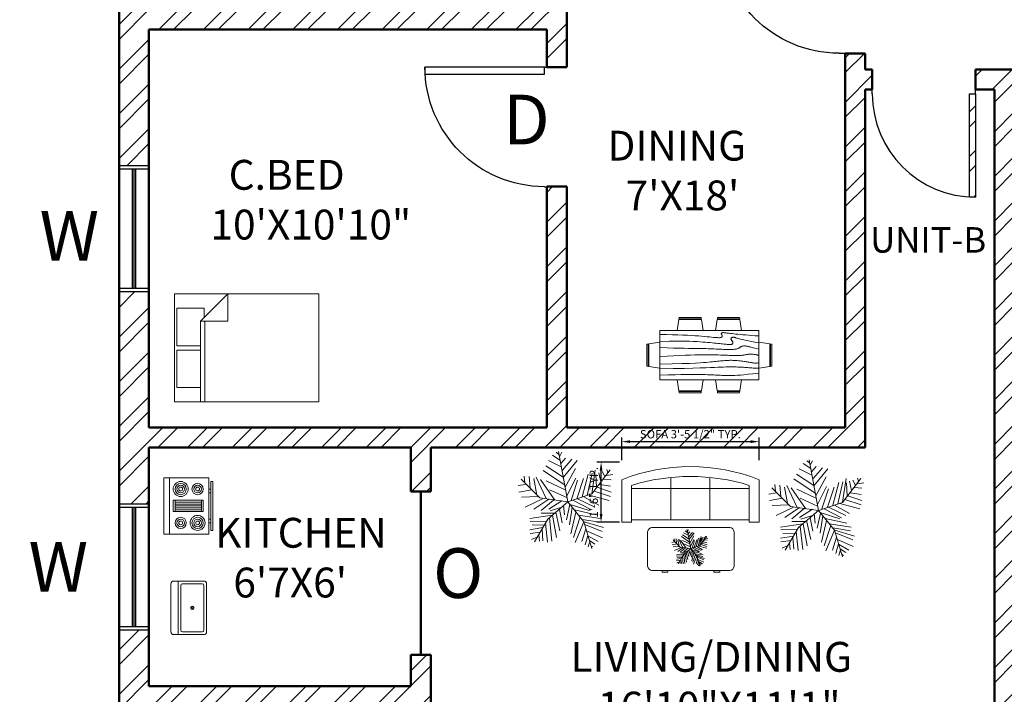
# Model space of a CAD drawing. Units: inches. Extents: x -31842 to -29388, y 18869 to 19743.
# Tile 6 of 12: x -30914 to -30617, y 19226 to 19429. Entities that reach past the tile are written whole.
import ezdxf

# ---------------------------------------------------------------- set-up
doc = ezdxf.new("R2010")
doc.units = ezdxf.units.IN
for name, color, linetype, lineweight in [('A-ANNO-DIMS', 2, 'Continuous', 18), ('A-ANNO-SYMB', 2, 'Continuous', 18), ('A-AREA-IDEN', 3, 'Continuous', 18), ('A-DOOR', 3, 'Continuous', 25), ('A-FLOR-FIXT', 8, 'Continuous', 18), ('A-FURN', 8, 'Continuous', 18), ('A-GLAZ', 4, 'Continuous', 25), ('A-WALL', 7, 'Continuous', 50), ('A-WALL-PATT', 8, 'Continuous', 13), ('L-PLNT', 3, 'Continuous', 13)]:
    doc.layers.add(name, color=color, linetype=linetype, lineweight=lineweight)
doc.styles.get("Standard").update_dxf_attribs({"font": 'arial.ttf'})
doc.dimstyles.new('ISO-25', dxfattribs={"dimtxt": 2.5, "dimasz": 2.5, "dimexe": 1.25, "dimexo": 0.625, "dimtad": 1, "dimdec": 0, "dimlunit": 3, "dimtxsty": 'Standard', "dimcen": 2.5, "dimadec": 0, "dimazin": 0, "dimtfac": 1, "dimtdec": 0, "dimtmove": 0, "dimatfit": 3, "dimfxl": 1, "dimarcsym": 0})

# ---------------------------------------------------------------- blocks, each defined once
blk = doc.blocks.new('*U8')
for p, q in [((0, 0), (0, -100)), ((750, 0), (750, -100))]:
    blk.add_line(p, q)
blk.add_lwpolyline([(0, 0), (0, 750), (43.75, 750), (43.75, 0)], close=True)
blk.add_arc((0, 0), 750, 0, 90)
blk = doc.blocks.new('Bed - Queen')
for p, q in [((0, -80.00003), (0, 0)), ((0, 0), (59.99999, 0)), ((59.99999, 0), (59.99999, -80.00003)), ((7.99999, -1.2), (28.79998, -1.2)), ((7.99999, -14.4), (7.99999, -1.2)), ((28.79998, -1.2), (28.79998, -14.4)), ((31.19999, -1.2), (51.99999, -1.2)), ((31.19999, -14.4), (31.19999, -1.2)), ((51.99999, -1.2), (51.99999, -16.4)), ((0, -14.4), (44.8, -14.4)), ((59.99999, -29.6), (44.8, -14.4)), ((44.8, -14.4), (44.8, -29.6)), ((44.8, -16.8), (0, -16.8)), ((51.99999, -16.4), (46.79936, -16.4)), ((44.8, -29.6), (59.99999, -29.6)), ((59.99999, -80.00003), (0, -80.00003))]:
    blk.add_line(p, q)
blk = doc.blocks.new('Range-Oven - 30 in top')
for p, q in [((0, -3), (30, -3)), ((12, -6), (18, -6)), ((13, -20), (13, -6)), ((14, -6), (14, -20)), ((15, -20), (15, -6)), ((16, -6), (16, -20)), ((17, -20), (17, -6)), ((18, -20), (12, -20)), ((6, -24), (6, -25)), ((8, -25), (8, -24)), ((22, -25), (22, -24)), ((24, -24), (24, -25))]:
    blk.add_line(p, q)
for points in [[(0, -24), (0, 0), (30, 0), (30, -24)], [(12, -21), (12, -5), (18, -5), (18, -21)], [(2, -26), (2, -25), (28, -25), (28, -26)]]:
    blk.add_lwpolyline(points, close=True)
for centre, radius in [((6, -9), 4), ((6, -9), 3), ((6, -9), 2), ((6, -9), 1), ((24, -9), 3), ((24, -9), 2), ((24, -9), 1), ((6, -18), 3), ((24, -18), 4), ((24, -18), 3), ((6, -18), 2), ((6, -18), 1), ((24, -18), 2), ((24, -18), 1)]:
    blk.add_circle(centre, radius)
blk = doc.blocks.new('Sink-single - 30 in top')
blk.add_line((-15, -3.999996), (15, -3.999996))
for points in [[(-13.5, 0), (13.5, 0)], [(-15, -18.499996), (-15, -1.5)], [(-12.5, -5.499996), (12.5, -5.499996)], [(15, -1.5), (15, -18.499996)], [(-13.5, -17.499996), (-13.5, -6.499996)], [(13.5, -6.499996), (13.5, -17.499996)], [(13.5, -19.999996), (-13.5, -19.999996)], [(12.5, -18.499996), (-12.5, -18.499996)]]:
    blk.add_lwpolyline(points)
for radius in [1, 0.5]:
    blk.add_circle((0, -11.999996), radius)
for centre, radius, start, end in [((-13.5, -1.5), 1.5, 90, 180), ((-12.5, -6.499996), 1, 90, 180), ((12.5, -6.499996), 1, 0, 90), ((13.5, -1.5), 1.5, 0, 90), ((-13.5, -18.499996), 1.5, 180, 270), ((-12.5, -17.499996), 1, 180, 270), ((12.5, -17.499996), 1, 270, 0), ((13.5, -18.499996), 1.5, 270, 0)]:
    blk.add_arc(centre, radius, start, end)
blk = doc.blocks.new('Desk - 30 x 60 in.')
for p, q in [((-26.999995, 0), (26.999995, 0)), ((-29.999995, -27), (-29.999995, -3)), ((29.999995, -3), (29.999995, -27)), ((26.999995, -30), (-26.999995, -30)), ((-20.000005, -30), (-20.000005, -31)), ((-20.000005, -31), (-16.000005, -31)), ((-16.000005, -31), (-16.000005, -30)), ((15.999995, -31), (15.999995, -30)), ((19.999995, -31), (15.999995, -31)), ((19.999995, -30), (19.999995, -31))]:
    blk.add_line(p, q)
for centre, start, end in [((-26.499995, -3.5), 98.1301, 171.8699), ((26.499995, -3.5), 8.130102, 81.8699), ((-26.499995, -26.5), 188.1301, 261.8699), ((26.499995, -26.5), 278.1301, 351.8699)]:
    blk.add_arc(centre, 3.535534, start, end)
blk = doc.blocks.new('Sofa - Roundback 7 ft.')
for p, q in [((-36.000027, -34), (-36.000027, -11.4696)), ((-12.00002, -32.4421), (-12.00003, -6.5971)), ((11.99997, -32.4421), (11.99998, -6.5971)), ((35.99998, -34), (35.99998, -11.4696)), ((-35.999844, -13.3819), (35.9998, -13.3819)), ((-36.000027, -32.4421), (35.99998, -32.4421))]:
    blk.add_line(p, q)
for points in [[(-36.000027, -34), (-42.000027, -34), (-42.000027, -8)], [(41.99998, -8), (41.99998, -34), (35.99998, -34)]]:
    blk.add_lwpolyline(points)
for centre, radius, start, end in [((0, -114.25), 114.25, 68.43141, 111.5686), ((-0.00001, -127.1968), 121.1968, 72.72033, 107.2797)]:
    blk.add_arc(centre, radius, start, end)
blk = doc.blocks.new('Dining Set - 36 x 72 in.')
for p, q in [((-22.2343, 26.00059), (-23.4847, 17.99762)), ((-22.2304, 26), (-5.7608, 26)), ((-22, 27.5), (-22.1562, 26.50042)), ((-5.8416, 26.5), (-22.1534, 26.5)), ((-22, 27.5), (-6, 27.5)), ((-5.8437, 26.49966), (-6, 27.5)), ((-4.5152, 17.99762), (-5.7655, 25.99926)), ((5.7657, 26.00059), (4.5153, 17.99762)), ((5.7696, 26), (22.2392, 26)), ((6, 27.5), (5.8438, 26.50042)), ((22.1584, 26.5), (5.8466, 26.5)), ((6, 27.5), (22, 27.5)), ((22.1563, 26.49966), (22, 27.5)), ((23.4848, 17.99762), (22.2345, 25.99926)), ((36, 18), (-36, 18)), ((-36, 18), (-36, -18)), ((36, -18), (36, 18)), ((-45.5, 8), (-44.5004, 8.15617)), ((-45.5, 8), (-45.5, -8)), ((-44.5, -8.15843), (-44.5, 8.15338)), ((-44.0006, 8.23428), (-35.9976, 9.48474)), ((-44, 8.23041), (-44, -8.23915)), ((44.0006, 8.23428), (35.9976, 9.48474)), ((44, 8.23041), (44, -8.23915)), ((44.5, -8.15843), (44.5, 8.15338)), ((45.5, 8), (44.5005, 8.15617)), ((45.5, 8), (45.5, -8)), ((-44.4997, -8.15631), (-45.5, -8)), ((-35.9976, -9.48476), (-43.9993, -8.2345)), ((35.9976, -9.48476), (43.9993, -8.2345)), ((44.4997, -8.15631), (45.5, -8)), ((-36, -18), (36, -18)), ((-22.2343, -26.0006), (-23.4847, -17.99762)), ((-4.5152, -17.99762), (-5.7655, -25.99928)), ((5.7657, -26.0006), (4.5153, -17.99762)), ((23.4848, -17.99762), (22.2345, -25.99928)), ((-22.2304, -26), (-5.7608, -26)), ((-22, -27.5), (-22.1562, -26.50044)), ((-5.8416, -26.5), (-22.1534, -26.5)), ((-22, -27.5), (-6, -27.5)), ((-5.8437, -26.49967), (-6, -27.5)), ((5.7696, -26), (22.2392, -26)), ((6, -27.5), (5.8438, -26.50044)), ((22.1584, -26.5), (5.8466, -26.5)), ((6, -27.5), (22, -27.5)), ((22.1563, -26.49967), (22, -27.5))]:
    blk.add_line(p, q)
for points in [[(-36, 15), (-31.1772, 14.97754), (-26.8079, 14.91406), (-22.8538, 14.81543), (-19.276, 14.6875), (-16.0362, 14.53613), (-13.0957, 14.36718), (-10.4159, 14.18652), (-7.9583, 14), (-5.6904, 13.81315), (-3.6035, 13.63021), (-1.6954, 13.45508), (0.0365, 13.29166), (1.5945, 13.14388), (2.9811, 13.01562), (4.1988, 12.9108), (5.25, 12.83333), (6.1393, 12.78613), (6.8802, 12.76823), (7.4883, 12.77767), (7.9792, 12.8125), (8.3685, 12.87077), (8.6719, 12.95052), (8.9049, 13.0498), (9.0833, 13.16666), (9.2205, 13.29899), (9.3216, 13.44401), (9.3895, 13.59879), (9.4271, 13.76041), (9.4373, 13.92594), (9.4232, 14.09245), (9.3875, 14.257), (9.3333, 14.41666), (9.2638, 14.56917), (9.1836, 14.71484), (9.0975, 14.85465), (9.0104, 14.98958), (8.9272, 15.1206), (8.8529, 15.2487), (8.7922, 15.37483), (8.75, 15.5), (8.7305, 15.62467), (8.7344, 15.74739), (8.7617, 15.86621), (8.8125, 15.97916), (8.8867, 16.08431), (8.9844, 16.17968), (9.1055, 16.26334), (9.25, 16.33333), (9.4189, 16.38802), (9.6172, 16.42708), (9.8506, 16.45052), (10.125, 16.45833), (10.4463, 16.45052), (10.8203, 16.42708), (11.2529, 16.38802), (11.75, 16.33333), (12.3184, 16.26318), (12.9694, 16.17838), (13.7151, 16.07991), (14.5677, 15.96875), (15.5395, 15.84586), (16.6426, 15.71224), (17.8893, 15.56884), (19.2917, 15.41666), (20.859, 15.25667), (22.5879, 15.08984), (24.4721, 14.91715), (26.5052, 14.73958), (28.6809, 14.5581), (30.9929, 14.3737), (33.4347, 14.18733), (36, 14)], [(-36, 10), (-28.9766, 10.14274), (-23.1725, 10.20442), (-18.4241, 10.19775), (-14.5677, 10.13541), (-11.4399, 10.03011), (-8.877, 9.89453), (-6.7154, 9.74137), (-4.7917, 9.58333), (-2.9698, 9.43082), (-1.2246, 9.28515), (0.4415, 9.14534), (2.026, 9.01041), (3.5266, 8.87939), (4.9408, 8.7513), (6.266, 8.62516), (7.5, 8.5), (8.6411, 8.37549), (9.6914, 8.2539), (10.6538, 8.13818), (11.5312, 8.03125), (12.3267, 7.93603), (13.043, 7.85547), (13.6831, 7.79248), (14.25, 7.75), (14.7471, 7.7303), (15.1797, 7.73307), (15.5537, 7.75732), (15.875, 7.80208), (16.1494, 7.86637), (16.3828, 7.94922), (16.5811, 8.04964), (16.75, 8.16666), (16.8944, 8.29915), (17.0143, 8.44531), (17.1089, 8.60319), (17.1771, 8.77083), (17.218, 8.94629), (17.2305, 9.1276), (17.2137, 9.31282), (17.1667, 9.5), (17.0895, 9.6875), (16.987, 9.875), (16.8649, 10.0625), (16.7292, 10.25), (16.5856, 10.4375), (16.4401, 10.625), (16.2985, 10.8125), (16.1667, 11), (16.05, 11.18733), (15.9518, 11.3737), (15.8752, 11.5581), (15.8229, 11.73958), (15.798, 11.91715), (15.8034, 12.08984), (15.842, 12.25667), (15.9167, 12.41666), (16.0295, 12.56836), (16.1784, 12.70833), (16.3605, 12.83268), (16.5729, 12.9375), (16.8127, 13.01888), (17.0768, 13.07291), (17.3625, 13.0957), (17.6667, 13.08333), (17.9894, 13.03312), (18.3418, 12.94726), (18.7382, 12.82918), (19.1927, 12.68229), (19.7195, 12.51001), (20.3327, 12.31575), (21.0465, 12.10294), (21.875, 11.875), (22.8357, 11.63354), (23.959, 11.37304), (25.2786, 11.08618), (26.8282, 10.76562), (28.6414, 10.40405), (30.752, 9.99414), (33.1936, 9.52856), (36, 9)], [(-36, 5.5), (-30.7157, 5.3348), (-26.069, 5.20963), (-21.9946, 5.11767), (-18.4271, 5.05208), (-15.3009, 5.00602), (-12.5508, 4.97265), (-10.1112, 4.94515), (-7.9167, 4.91666), (-5.909, 4.88167), (-4.0586, 4.83984), (-2.3429, 4.79215), (-0.7396, 4.73958), (0.7739, 4.6831), (2.22, 4.6237), (3.6213, 4.56233), (5, 4.5), (6.373, 4.43782), (7.7344, 4.3776), (9.0723, 4.32129), (10.375, 4.27083), (11.6309, 4.22819), (12.8281, 4.19531), (13.9551, 4.17415), (15, 4.16666), (15.954, 4.17448), (16.819, 4.19791), (17.6001, 4.23698), (18.3021, 4.29166), (18.9299, 4.36198), (19.4883, 4.44791), (19.9823, 4.54948), (20.4167, 4.66666), (20.7969, 4.79899), (21.1302, 4.94401), (21.4245, 5.09879), (21.6875, 5.26041), (21.9271, 5.42594), (22.1511, 5.59245), (22.3672, 5.757), (22.5834, 5.91666), (22.8065, 6.06868), (23.0404, 6.21093), (23.2879, 6.34147), (23.5521, 6.45833), (23.8358, 6.55957), (24.142, 6.64323), (24.4735, 6.70735), (24.8334, 6.75), (25.2235, 6.76969), (25.642, 6.76692), (26.0858, 6.74267), (26.5521, 6.69791), (27.0379, 6.63362), (27.5404, 6.55078), (28.0565, 6.45036), (28.5834, 6.33333), (29.1242, 6.19987), (29.7071, 6.04687), (30.3661, 5.87044), (31.1354, 5.66666), (32.0493, 5.43164), (33.142, 5.16146), (34.4475, 4.85221), (36, 4.5)], [(-36, -1), (-30.7915, -0.6591), (-26.0195, -0.38216), (-21.6519, -0.16284), (-17.6563, 0.00521), (-14.0005, 0.12833), (-10.6523, 0.21289), (-7.5796, 0.26522), (-4.75, 0.29166), (-2.134, 0.29793), (0.2878, 0.28711), (2.5317, 0.26163), (4.6146, 0.22396), (6.5529, 0.17651), (8.3633, 0.12174), (10.0623, 0.06209), (11.6667, 0), (13.1899, -0.06201), (14.6341, -0.1211), (15.9982, -0.17432), (17.2813, -0.21875), (18.4823, -0.25147), (19.6003, -0.26953), (20.6343, -0.27002), (21.5834, -0.25), (22.4481, -0.20768), (23.2357, -0.14584), (23.9549, -0.06836), (24.6146, 0.02083), (25.2235, 0.11784), (25.7904, 0.21875), (26.3241, 0.31966), (26.8334, 0.41666), (27.3265, 0.50618), (27.8099, 0.58593), (28.2894, 0.65397), (28.7709, 0.70833), (29.2601, 0.74707), (29.763, 0.76823), (30.2855, 0.76985), (30.8334, 0.75), (31.4088, 0.70784), (31.9994, 0.64713), (32.589, 0.57275), (33.1615, 0.48958), (33.7008, 0.4025), (34.1908, 0.3164), (34.6153, 0.23616), (34.9584, 0.16666), (35.2099, 0.11165), (35.3848, 0.07031), (35.504, 0.04069), (35.5886, 0.02083), (35.6594, 0.00879), (35.7377, 0.0026), (35.8442, 0.00032), (36, 0)], [(-36, -6.5), (-27.1843, -6.31267), (-20.084, -6.1263), (-14.469, -5.9419), (-10.1094, -5.76042), (-6.7752, -5.58285), (-4.2363, -5.41016), (-2.2629, -5.24333), (-0.625, -5.08334), (0.8708, -4.93099), (2.2715, -4.78646), (3.5872, -4.64974), (4.8281, -4.52084), (6.0046, -4.39974), (7.127, -4.28646), (8.2053, -4.18099), (9.25, -4.08334), (10.2705, -3.99382), (11.2734, -3.91407), (12.2647, -3.84603), (13.25, -3.79167), (14.2354, -3.75293), (15.2266, -3.73177), (16.2295, -3.73015), (17.25, -3.75), (18.2912, -3.79248), (19.3451, -3.85547), (20.4009, -3.93604), (21.4479, -4.03125), (22.4754, -4.13819), (23.4727, -4.25391), (24.4289, -4.37549), (25.3334, -4.5), (26.1785, -4.62492), (26.9694, -4.74935), (27.7145, -4.87281), (28.4219, -4.99479), (29.1, -5.11483), (29.7572, -5.23242), (30.4016, -5.34709), (31.0417, -5.45834), (31.6837, -5.56437), (32.3262, -5.65821), (32.9658, -5.73153), (33.599, -5.77604), (34.2224, -5.78345), (34.8327, -5.74545), (35.4264, -5.65373), (36, -5.5)], [(-36, -10), (-26.4022, -9.81299), (-18.4675, -9.62891), (-11.9839, -9.45069), (-6.7396, -9.28125), (-2.5226, -9.12354), (0.8789, -8.98047), (3.6769, -8.85498), (6.0833, -8.75), (8.2767, -8.66765), (10.3021, -8.60677), (12.1712, -8.56543), (13.8958, -8.54167), (15.4876, -8.53353), (16.9583, -8.53907), (18.3197, -8.55632), (19.5834, -8.58334), (20.7616, -8.61841), (21.8685, -8.66081), (22.9188, -8.71004), (23.9271, -8.76563), (24.9081, -8.82707), (25.8763, -8.89388), (26.8465, -8.96558), (27.8334, -9.04167), (28.8474, -9.12118), (29.8828, -9.20117), (30.93, -9.27824), (31.9792, -9.34896), (33.0205, -9.40991), (34.0443, -9.45768), (35.0407, -9.48885), (36, -9.5)], [(-36, -14.5), (-30.0881, -14.33513), (-25.0332, -14.21224), (-20.7312, -14.12647), (-17.0781, -14.07292), (-13.97, -14.04671), (-11.3027, -14.04297), (-8.9724, -14.05681), (-6.875, -14.08334), (-4.9224, -14.11833), (-3.0905, -14.16016), (-1.3709, -14.20785), (0.2448, -14.26042), (1.7647, -14.3169), (3.1973, -14.3763), (4.5507, -14.43767), (5.8333, -14.5), (7.0554, -14.5621), (8.235, -14.62175), (9.3922, -14.67652), (10.5469, -14.72396), (11.7192, -14.76164), (12.929, -14.78711), (14.1965, -14.79794), (15.5417, -14.79167), (16.9933, -14.76424), (18.6152, -14.70508), (20.4804, -14.60197), (22.6615, -14.44271), (25.2312, -14.21509), (28.2624, -13.9069), (31.8277, -13.50594), (36, -13)]]:
    blk.add_lwpolyline(points)
blk = doc.blocks.new('*U122')
for p, q in [((-258.7244, 1362.456), (-332.3336, 1421.4348)), ((0, 0), (-266.7, 1447.8)), ((-231.1146, 1315.2628), (-166.7002, 1421.4348)), ((-185.1152, 1008.5578), (-553.1612, 1185.4942)), ((-221.9198, 1197.3052), (-433.5526, 1338.8594)), ((-194.31, 1102.9442), (-65.4812, 1256.284)), ((-148.3106, 914.1968), (118.5418, 1220.9018)), ((-129.8956, 701.8528), (265.7602, 1185.4942)), ((-93.091, 489.5342), (-700.3796, 902.3858)), ((-129.8956, 713.6638), (-626.7704, 1032.1544)), ((-74.7014, 418.7444), (219.7608, 961.39)), ((685.8, 228.6), (1219.2, 914.4)), ((689.0258, 230.0224), (790.2448, 914.1968)), ((983.4626, 867.0036), (1066.2666, 725.4494)), ((1121.4862, 925.9824), (1149.0706, 831.6214)), ((-800.1, 114.3), (-1333.5, 647.7)), ((-1234.059, 536.7274), (-1252.4486, 737.2604)), ((-1105.2302, 725.4494), (-1077.6458, 395.1732)), ((-976.4268, 666.4706), (-884.4026, 194.6402)), ((-902.8176, 713.6638), (-617.5756, 100.2538)), ((-369.1382, 53.086), (-783.1836, 642.874)), ((-617.5756, 607.4918), (-74.7014, 347.98)), ((-28.6766, 171.0436), (228.9556, 678.2816)), ((100.1268, 41.275), (284.1498, 619.2774)), ((256.5654, 88.4682), (449.7832, 666.4706)), ((412.9786, 147.447), (587.8068, 796.2392)), ((560.197, 182.8292), (698.2206, 819.8358)), ((808.6344, 784.4282), (827.0494, 418.7444)), ((891.4384, 831.6214), (946.658, 572.1096)), ((1029.462, 654.685), (1241.0948, 631.0884)), ((1112.2914, 760.8316), (1296.3144, 784.4282)), ((-1206.4492, 501.3198), (-1418.082, 465.9376)), ((-1031.621, 347.98), (-1399.667, 277.1902)), ((-525.5514, 347.98), (-28.6766, 123.8504)), ((753.4148, 312.5978), (1222.6798, 159.2326)), ((845.439, 418.7444), (1241.0948, 277.1902)), ((919.0482, 501.3198), (1222.6798, 454.152)), ((-847.598, 159.2326), (-1326.0578, 135.636)), ((-718.7946, 88.4682), (-1215.644, -147.447)), ((-543.9664, 76.6572), (-967.2066, -206.4512)), ((0, 0), (-800.1, 114.3)), ((-405.9428, 53.086), (-764.794, -241.8334)), ((0, 0), (-571.5, -495.3)), ((-166.7002, 29.4894), (-543.9664, -206.4512)), ((0, 0), (685.8, 228.6)), ((0, 0), (457.2, -571.5)), ((164.5412, 41.275), (661.416, -218.2368)), ((284.1498, 88.4682), (781.0246, -147.447)), ((458.978, 147.447), (891.4384, -88.4682)), ((615.4166, 194.6402), (1185.8752, 41.275)), ((-166.7002, -147.447), (-507.1618, -253.619)), ((-240.3094, -218.2368), (-157.5054, -595.7062)), ((-120.7008, -88.4682), (-93.091, -371.5766)), ((63.3222, -76.6826), (-37.8714, -513.1308)), ((44.9326, -64.897), (615.4166, -241.8334)), ((127.7366, -159.258), (54.1274, -654.685)), ((192.151, -230.0224), (817.8292, -371.5766)), ((-442.7474, -383.3876), (-1086.8406, -477.7486)), ((-617.5756, -548.5384), (-1077.6458, -560.324)), ((-571.5, -495.3), (-952.5, -1143)), ((-387.5278, -324.4088), (-764.794, -324.4088)), ((-525.5514, -465.963), (-451.9422, -1126.5408)), ((-433.5526, -383.3876), (-323.1134, -1020.3688)), ((-341.5284, -289.0012), (-221.9198, -831.6214)), ((228.9556, -289.0012), (90.932, -914.1968)), ((357.759, -430.5554), (164.5412, -1020.3688)), ((311.7596, -383.3876), (937.4378, -477.7486)), ((412.9786, -501.3452), (919.0482, -583.9206)), ((-718.7946, -737.2604), (-1086.8406, -796.2392)), ((-681.9646, -666.496), (-1022.4262, -654.685)), ((-737.1842, -784.4536), (-709.5744, -1114.7298)), ((-635.9652, -607.5172), (-580.771, -1150.1374)), ((458.978, -572.1096), (210.5406, -1161.923)), ((514.1976, -772.6426), (403.7838, -1138.3264)), ((457.2, -571.5), (685.8, -1333.5)), ((468.1982, -572.1096), (1029.462, -737.2604)), ((486.5878, -642.8994), (983.4626, -843.4324)), ((541.8074, -831.6214), (992.6574, -1032.1544)), ((-783.1836, -867.029), (-1077.6458, -902.4112)), ((-875.2078, -1008.5832), (-1040.8412, -1079.3476)), ((-829.2084, -937.7934), (-810.7934, -1126.5408)), ((578.612, -961.39), (495.7826, -1232.7128)), ((578.612, -973.1756), (873.0488, -1138.3264)), ((624.6114, -1102.9442), (781.0246, -1209.1162)), ((624.6114, -1161.923), (587.8068, -1291.6916)), ((679.8056, -1268.095), (716.6102, -1291.6916))]:
    blk.add_line(p, q)
blk = doc.blocks.new('WIN-3FT')
for p, q in [((0, 36), (9, 36)), ((4, 0), (4, 36)), ((4.5, 0), (4.5, 36)), ((5, 0), (5, 36)), ((0, 0), (9, 0))]:
    blk.add_line(p, q)
blk = doc.blocks.new('*D255')
at = {"layer": 'A-ANNO-DIMS', "color": 0, "lineweight": -2, "transparency": 16777216}
for p, q in [((-30732.8, 19296.13), (-30732.8, 19302.97)), ((-30691.37, 19296.13), (-30691.37, 19302.97)), ((-30730.3, 19301.72), (-30693.87, 19301.72))]:
    blk.add_line(p, q, dxfattribs=at)
at = {"layer": 'A-ANNO-DIMS', "color": 0, "transparency": 16777216}
for points in [[(-30730.3, 19302.14), (-30730.3, 19301.31), (-30732.8, 19301.72)], [(-30693.87, 19302.14), (-30693.87, 19301.31), (-30691.37, 19301.72)]]:
    blk.add_solid(points, dxfattribs=at)
at = {"layer": 'Defpoints', "color": 0, "transparency": 16777216}
for p in [(-30691.37, 19301.72), (-30732.8, 19295.51), (-30691.37, 19295.51)]:
    blk.add_point(p, dxfattribs=at)
at = {"layer": 'A-ANNO-DIMS', "color": 0, "transparency": 16777216, "insert": (-30712.09, 19303.64), "char_height": 2.5, "attachment_point": 5}
blk.add_mtext('SOFA 3\'-5 1/2" TYP.', dxfattribs=at)
blk = doc.blocks.new('*D256')
at = {"layer": 'A-ANNO-DIMS', "color": 0, "lineweight": -2, "transparency": 16777216}
for p, q in [((-30733.43, 19295.51), (-30740.27, 19295.51)), ((-30739.02, 19279.92), (-30739.02, 19293.01)), ((-30733.43, 19277.42), (-30740.27, 19277.42))]:
    blk.add_line(p, q, dxfattribs=at)
at = {"layer": 'A-ANNO-DIMS', "color": 0, "transparency": 16777216}
for points in [[(-30739.44, 19293.01), (-30738.6, 19293.01), (-30739.02, 19295.51)], [(-30739.44, 19279.92), (-30738.6, 19279.92), (-30739.02, 19277.42)]]:
    blk.add_solid(points, dxfattribs=at)
at = {"layer": 'Defpoints', "color": 0, "transparency": 16777216}
for p in [(-30739.02, 19295.51), (-30732.8, 19295.51), (-30732.8, 19277.42)]:
    blk.add_point(p, dxfattribs=at)
at = {"layer": 'A-ANNO-DIMS', "color": 0, "transparency": 16777216, "insert": (-30740.92, 19286.47), "char_height": 2.5, "attachment_point": 5, "rotation": 90}
blk.add_mtext('1\'-6" TYP.', dxfattribs=at)

msp = doc.modelspace()

# ---------------------------------------------------------------- hatches: boundary and pattern name
at = {"layer": 'A-WALL-PATT'}
h = msp.add_hatch(dxfattribs=at)
h.set_pattern_fill('ANSI32', color=256)
h.paths.add_polyline_path([(-30352.39, 19656.96), (-30487.39, 19656.96), (-30487.39, 19614.96), (-30510.39, 19614.96), (-30510.39, 19605.96), (-30487.39, 19605.96), (-30487.39, 19558.38), (-30481.39, 19558.38), (-30481.39, 19605.96), (-30469.68, 19605.96), (-30469.68, 19614.96), (-30481.39, 19614.96), (-30481.39, 19650.96), (-30361.39, 19650.96), (-30361.39, 19614.96), (-30445.68, 19614.96), (-30445.68, 19605.96), (-30361.39, 19605.96), (-30361.39, 19564.96), (-30352.39, 19564.96)])
h.paths.add_polyline_path([(-30548.39, 19614.96), (-30599.39, 19614.96), (-30599.39, 19605.96), (-30577.39, 19605.96), (-30577.39, 19457.87), (-30571.39, 19457.87), (-30571.39, 19491.96), (-30560.76, 19491.96), (-30560.76, 19497.96), (-30571.39, 19497.96), (-30571.39, 19605.96), (-30548.39, 19605.96)])
h.paths.add_polyline_path([(-30637.39, 19614.96), (-30688.39, 19614.96), (-30688.39, 19605.96), (-30665.39, 19605.96), (-30665.39, 19497.96), (-30682.48, 19497.96), (-30682.48, 19491.96), (-30665.39, 19491.96), (-30665.39, 19454.79), (-30662.43, 19454.79), (-30659.39, 19454.79), (-30659.39, 19605.96), (-30637.39, 19605.96)])
h.paths.add_polyline_path([(-30789.63, 19614.96), (-30875.39, 19614.96), (-30875.39, 19650.96), (-30755.39, 19650.96), (-30755.39, 19614.96), (-30765.63, 19614.96), (-30765.63, 19605.96), (-30755.39, 19605.96), (-30755.39, 19550.68), (-30749.39, 19550.68), (-30749.39, 19605.96), (-30726.39, 19605.96), (-30726.39, 19614.96), (-30749.39, 19614.96), (-30749.39, 19656.96), (-30884.39, 19656.96), (-30884.39, 19564.96), (-30875.39, 19564.96), (-30875.39, 19605.96), (-30789.63, 19605.96)])
h.paths.add_polyline_path([(-30749.39, 19491.96), (-30736.92, 19491.96), (-30736.92, 19494.96), (-30682.48, 19494.96), (-30682.48, 19497.96), (-30665.39, 19497.96), (-30665.39, 19605.96), (-30688.39, 19605.96), (-30749.39, 19605.96), (-30749.39, 19550.68), (-30755.39, 19550.68), (-30757.34, 19550.71, 0.39722), (-30793.34, 19516.76), (-30757.34, 19516.76), (-30757.34, 19514.65), (-30793.4, 19514.65), (-30793.4, 19516.76), (-30793.34, 19516.76, -0.39722), (-30757.34, 19550.71), (-30755.39, 19550.71), (-30755.39, 19605.96), (-30765.63, 19605.96), (-30765.63, 19613.66), (-30767.03, 19613.66), (-30767.03, 19637.62, 0.397344), (-30789.63, 19613.65), (-30789.63, 19605.96), (-30875.39, 19605.96), (-30875.39, 19564.96), (-30875.39, 19485.96), (-30873.79, 19485.96), (-30873.79, 19479.96), (-30873.79, 19479.35, 0.39722), (-30851.19, 19455.39), (-30851.19, 19479.35), (-30849.79, 19479.35), (-30849.79, 19455.34), (-30851.19, 19455.34), (-30851.19, 19455.39, -0.39722), (-30873.79, 19479.35), (-30873.79, 19479.96), (-30875.39, 19479.96), (-30875.39, 19431.96), (-30848.39, 19431.96), (-30848.39, 19468.96), (-30842.39, 19468.96), (-30842.39, 19479.96), (-30755.39, 19479.96), (-30755.39, 19470.97), (-30749.39, 19470.97)])
h.paths.add_polyline_path([(-30738.39, 19585.51), (-30738.39, 19586.08), (-30736.12, 19586.08), (-30736.12, 19586.65), (-30739.53, 19586.65), (-30739.53, 19600.27), (-30722.5, 19600.27), (-30722.5, 19586.65), (-30725.91, 19586.65), (-30725.91, 19586.08), (-30723.64, 19586.08), (-30723.64, 19585.51)], flags=16)
h.paths.add_polyline_path([(-30737.83, 19590.05, -1), (-30734.42, 19590.05, -1)], flags=16)
h.paths.add_polyline_path([(-30737.26, 19590.05, -1), (-30734.99, 19590.05, -1)], flags=0)
h.paths.add_polyline_path([(-30732.72, 19588.35), (-30732.72, 19597.43), (-30729.31, 19597.43), (-30729.31, 19588.35)], flags=16)
h.paths.add_polyline_path([(-30736.69, 19590.05, -1), (-30735.56, 19590.05, -1)], flags=0)
h.paths.add_polyline_path([(-30732.15, 19588.92), (-30732.15, 19596.86), (-30729.88, 19596.86), (-30729.88, 19588.92)], flags=0)
h.paths.add_polyline_path([(-30728.18, 19590.05, -1), (-30723.64, 19590.05, -1)], flags=0)
h.paths.add_polyline_path([(-30727.61, 19590.05, -1), (-30724.2, 19590.05, -1)], flags=0)
h.paths.add_polyline_path([(-30727.04, 19590.05, -1), (-30724.77, 19590.05, -1)], flags=0)
h.paths.add_polyline_path([(-30726.47, 19590.05, -1), (-30725.34, 19590.05, -1)], flags=0)
h.paths.add_polyline_path([(-30738.39, 19595.16, -1), (-30733.85, 19595.16, -1)], flags=16)
h.paths.add_polyline_path([(-30737.83, 19595.16, -1), (-30734.42, 19595.16, -1)], flags=0)
h.paths.add_polyline_path([(-30737.26, 19595.16, -1), (-30734.99, 19595.16, -1)], flags=0)
h.paths.add_polyline_path([(-30736.69, 19595.16, -1), (-30735.56, 19595.16, -1)], flags=0)
h.paths.add_polyline_path([(-30727.61, 19595.16, -1), (-30724.2, 19595.16, -1)], flags=0)
h.paths.add_polyline_path([(-30727.04, 19595.16, -1), (-30724.77, 19595.16, -1)], flags=0)
h.paths.add_polyline_path([(-30707.55, 19587.34, -0.414214), (-30708.36, 19588.14), (-30708.36, 19597.29, -0.414214), (-30707.55, 19598.09), (-30693.03, 19598.09, -0.414214), (-30692.23, 19597.29), (-30692.23, 19588.14, -0.414214), (-30693.03, 19587.34)], flags=16)
h.paths.add_polyline_path([(-30726.47, 19595.16, -1), (-30725.34, 19595.16, -1)], flags=0)
h.paths.add_polyline_path([(-30827.74, 19570.11), (-30871.22, 19570.11), (-30871.22, 19602.72), (-30827.74, 19602.72)], flags=16)
h.paths.add_polyline_path([(-30707.01, 19588.14, -0.414214), (-30707.55, 19588.68), (-30707.55, 19594.6, -0.414214), (-30707.01, 19595.13), (-30693.57, 19595.13, -0.414214), (-30693.03, 19594.6), (-30693.03, 19588.68, -0.414214), (-30693.57, 19588.14)], flags=0)
h.paths.add_polyline_path([(-30700.02, 19591.64, -1), (-30700.56, 19591.64, -1)], flags=0)
h.paths.add_polyline_path([(-30863.39, 19594.46), (-30863.39, 19574.46), (-30870.57, 19574.46), (-30870.57, 19585.76), (-30863.39, 19585.76), (-30863.39, 19587.07), (-30870.57, 19587.07), (-30870.57, 19598.37), (-30862.31, 19598.37), (-30862.31, 19595.55), (-30855.13, 19602.72), (-30855.13, 19594.46)], flags=0)
h.paths.add_polyline_path([(-30755.39, 19514.65), (-30757.34, 19514.65), (-30793.4, 19514.65), (-30793.4, 19516.76), (-30793.34, 19516.76, -0.39722), (-30757.34, 19550.71), (-30755.39, 19550.71), (-30755.39, 19605.96), (-30765.63, 19605.96), (-30765.63, 19613.66), (-30767.03, 19613.66), (-30767.03, 19637.62, 0.397344), (-30789.63, 19613.65), (-30789.63, 19605.96), (-30875.39, 19605.96), (-30875.39, 19564.96), (-30875.39, 19485.96), (-30873.79, 19485.96), (-30873.79, 19479.96), (-30873.79, 19479.35, 0.39722), (-30851.19, 19455.39), (-30851.19, 19479.35), (-30849.79, 19479.35), (-30849.79, 19479.96), (-30849.79, 19479.96), (-30849.79, 19485.96), (-30755.39, 19485.96)], flags=16)
h.paths.add_polyline_path([(-30665.39, 19605.96), (-30688.39, 19605.96), (-30749.39, 19605.96), (-30749.39, 19550.68), (-30755.39, 19550.68), (-30757.34, 19550.71, 0.39722), (-30793.34, 19516.76), (-30757.34, 19516.76), (-30757.34, 19514.65), (-30755.39, 19514.65), (-30755.39, 19514.68), (-30749.39, 19514.68), (-30749.39, 19497.96), (-30736.92, 19497.96), (-30736.92, 19494.96), (-30682.48, 19494.96), (-30682.48, 19497.96), (-30665.39, 19497.96)], flags=17)
h.paths.add_polyline_path([(-30749.39, 19446.97), (-30755.39, 19446.97), (-30755.39, 19431.96), (-30842.39, 19431.96), (-30842.39, 19442.96), (-30848.39, 19442.96), (-30848.39, 19431.96), (-30875.39, 19431.96), (-30875.39, 19479.96), (-30873.79, 19479.96), (-30873.79, 19482.55), (-30873.79, 19485.96), (-30875.39, 19485.96), (-30875.39, 19526.96), (-30884.39, 19526.96), (-30884.39, 19384.96), (-30875.39, 19384.96), (-30875.39, 19425.96), (-30755.39, 19425.96), (-30755.39, 19414.67), (-30751.3, 19414.67), (-30749.39, 19414.62)])
h.paths.add_polyline_path([(-30848.39, 19468.96), (-30848.39, 19479.96), (-30849.79, 19479.96), (-30849.79, 19479.35), (-30849.79, 19455.34), (-30851.19, 19455.34), (-30851.19, 19455.39, -0.39722), (-30873.79, 19479.35), (-30873.79, 19479.96), (-30875.39, 19479.96), (-30875.39, 19431.96), (-30848.39, 19431.96), (-30848.39, 19442.96)], flags=17)
h.paths.add_polyline_path([(-30659.39, 19407.96), (-30657.22, 19407.96), (-30657.22, 19413.96), (-30659.39, 19413.96), (-30659.39, 19418.79), (-30665.39, 19418.79), (-30665.39, 19305.96), (-30749.39, 19305.96), (-30749.39, 19378.62), (-30755.39, 19378.62), (-30755.39, 19305.96), (-30875.39, 19305.96), (-30875.39, 19346.96), (-30884.39, 19346.96), (-30884.39, 19282.96), (-30875.39, 19282.96), (-30875.39, 19299.96), (-30796.39, 19299.96), (-30796.39, 19286.68), (-30790.39, 19286.68), (-30790.39, 19299.96), (-30659.39, 19299.96)])
h.paths.add_polyline_path([(-30352.39, 19346.96), (-30361.39, 19346.96), (-30361.39, 19305.96), (-30481.39, 19305.96), (-30481.39, 19380.1), (-30487.39, 19380.1), (-30487.39, 19305.96), (-30571.39, 19305.96), (-30571.39, 19421.87), (-30577.39, 19421.87), (-30577.39, 19413.96), (-30579.53, 19413.96), (-30579.53, 19407.96), (-30577.39, 19407.96), (-30577.39, 19299.96), (-30446.39, 19299.96), (-30446.39, 19291.76), (-30440.39, 19291.76), (-30440.39, 19299.96), (-30361.39, 19299.96), (-30361.39, 19282.96), (-30352.39, 19282.96)])
h.paths.add_polyline_path([(-30481.39, 19449.62), (-30484.39, 19449.62), (-30487.39, 19449.62), (-30487.39, 19416.1), (-30481.39, 19416.1), (-30481.39, 19425.96), (-30361.39, 19425.96), (-30361.39, 19384.96), (-30352.39, 19384.96), (-30352.39, 19526.96), (-30361.39, 19526.96), (-30361.39, 19485.96), (-30363.32, 19485.96), (-30363.32, 19479.96), (-30361.39, 19479.96), (-30361.39, 19431.96), (-30388.39, 19431.96), (-30388.39, 19442.96), (-30394.39, 19442.96), (-30394.39, 19431.96), (-30481.39, 19431.96)])
h.paths.add_polyline_path([(-30387.32, 19482.76), (-30387.32, 19485.96), (-30481.39, 19485.96), (-30481.39, 19522.38), (-30487.39, 19522.38), (-30487.39, 19497.96), (-30500.08, 19497.96), (-30500.08, 19491.96), (-30487.39, 19491.96), (-30487.39, 19473.62), (-30481.39, 19473.62), (-30481.39, 19479.96), (-30394.39, 19479.96), (-30394.39, 19468.96), (-30388.39, 19468.96), (-30388.39, 19479.96), (-30387.32, 19479.96)])
h.paths.add_polyline_path([(-30626.04, 19413.96), (-30610.58, 19413.96), (-30610.58, 19407.24), (-30608.81, 19407.24), (-30608.81, 19376.14), (-30610.63, 19376.14), (-30610.63, 19407.96), (-30614.39, 19407.96), (-30614.39, 19173.96), (-30532.79, 19173.96), (-30532.79, 19167.96), (-30532.79, 19166.59), (-30532.79, 19167.96), (-30614.39, 19167.96), (-30614.39, 19023.96), (-30568.89, 19023.96), (-30568.89, 19014.96), (-30666.89, 19014.96), (-30666.89, 19018.96), (-30702.89, 19018.96), (-30702.89, 19019.96), (-30666.89, 19019.96), (-30666.89, 19023.96), (-30620.39, 19023.96), (-30620.39, 19167.96), (-30707.45, 19167.96), (-30707.45, 19166.65, -0.39722), (-30741.49, 19130.57), (-30741.49, 19130.51), (-30743.6, 19130.51), (-30743.6, 19166.65), (-30741.49, 19166.65), (-30741.49, 19130.57, 0.407721), (-30707.48, 19167.96), (-30707.53, 19167.96), (-30707.53, 19173.96), (-30620.39, 19173.96), (-30620.39, 19407.96), (-30626.04, 19407.96), (-30626.04, 19406.62), (-30626.04, 19375.45), (-30627.86, 19375.45), (-30627.86, 19406.62), (-30626.04, 19406.62), (-30626.04, 19407.96), (-30626.04, 19407.96)])
h.paths.add_polyline_path([(-30481.39, 19167.96), (-30478.24, 19167.96), (-30478.24, 19173.96), (-30487.39, 19173.96), (-30496.79, 19173.96), (-30496.79, 19167.96), (-30487.39, 19167.96), (-30487.39, 19023.96), (-30531.89, 19023.96), (-30531.89, 19014.96), (-30449.39, 19014.96), (-30449.39, 19023.96), (-30481.39, 19023.96)])
h.paths.add_polyline_path([(-30322.39, 19173.96), (-30343.77, 19173.96), (-30343.77, 19167.96), (-30328.39, 19167.96), (-30328.39, 19023.96), (-30373.39, 19023.96), (-30373.39, 19076.96), (-30379.39, 19076.96), (-30379.39, 19023.96), (-30411.39, 19023.96), (-30411.39, 19014.96), (-30322.39, 19014.96)])
h.paths.add_polyline_path([(-30367.77, 19173.96), (-30440.39, 19173.96), (-30440.39, 19191.96), (-30446.39, 19191.96), (-30446.39, 19173.96), (-30449.24, 19173.96), (-30449.24, 19167.96), (-30379.39, 19167.96), (-30379.39, 19114.96), (-30373.39, 19114.96), (-30373.39, 19167.96), (-30367.77, 19167.96)])
h.paths.add_polyline_path([(-30857.39, 19167.96), (-30814.74, 19167.96), (-30787.91, 19167.96), (-30787.91, 19173.96), (-30790.39, 19173.96), (-30790.39, 19191.02), (-30796.39, 19191.02), (-30796.39, 19173.96), (-30814.74, 19173.96), (-30871.78, 19173.96), (-30871.78, 19167.96), (-30863.39, 19167.96), (-30863.39, 19114.96), (-30857.39, 19114.96)])
h.paths.add_polyline_path([(-30857.39, 19076.96), (-30863.39, 19076.96), (-30863.39, 19023.96), (-30908.39, 19023.96), (-30908.39, 19167.96), (-30895.78, 19167.96), (-30895.78, 19173.96), (-30914.39, 19173.96), (-30914.39, 19014.96), (-30825.39, 19014.96), (-30825.39, 19023.96), (-30857.39, 19023.96)])
h.paths.add_polyline_path([(-30758.91, 19173.96), (-30743.53, 19173.96), (-30743.53, 19167.96), (-30743.6, 19166.65), (-30741.49, 19166.65), (-30741.49, 19130.51), (-30743.6, 19130.51), (-30743.6, 19166.65), (-30743.6, 19167.96), (-30749.39, 19167.96), (-30749.39, 19023.96), (-30702.89, 19023.96), (-30702.89, 19019.46), (-30666.89, 19019.46), (-30666.89, 19018.96), (-30702.89, 19018.96), (-30702.89, 19014.96), (-30788.39, 19014.96), (-30788.39, 19018.96), (-30824.39, 19018.96), (-30824.39, 19019.96), (-30788.39, 19019.96), (-30788.39, 19023.96), (-30755.39, 19023.96), (-30755.39, 19167.96), (-30758.91, 19167.96), (-30758.91, 19166.97), (-30758.91, 19137.97), (-30760.6, 19137.97), (-30760.6, 19166.97), (-30758.91, 19166.97), (-30758.91, 19167.96), (-30758.91, 19167.96)])
h.paths.add_polyline_path([(-30790.39, 19237.4), (-30796.39, 19237.4), (-30796.39, 19227.96), (-30875.39, 19227.96), (-30875.39, 19244.96), (-30884.39, 19244.96), (-30884.39, 19210.96), (-30875.39, 19210.96), (-30875.39, 19221.96), (-30796.39, 19221.96), (-30796.39, 19215.02), (-30793.87, 19215.02), (-30790.39, 19215.02)])
h.paths.add_polyline_path([(-30352.39, 19244.96), (-30361.39, 19244.96), (-30361.39, 19227.96), (-30440.39, 19227.96), (-30440.39, 19236.96), (-30446.39, 19236.96), (-30446.39, 19215.96), (-30440.39, 19215.96), (-30440.39, 19221.96), (-30361.39, 19221.96), (-30361.39, 19210.96), (-30352.39, 19210.96)])
h.paths.add_polyline_path([(-30788.99, 19602.36), (-30766.36, 19602.36), (-30766.36, 19633.27), (-30788.99, 19633.27)], flags=24)
h.paths.add_polyline_path([(-30871.43, 19460.05), (-30848.8, 19460.05), (-30848.8, 19490.96), (-30871.43, 19490.96)], flags=24)
h.paths.add_polyline_path([(-30778.82, 19519.23), (-30756.18, 19519.23), (-30756.18, 19550.14), (-30778.82, 19550.14)], flags=24)
h.paths.add_polyline_path([(-30741.54, 19533.68), (-30681.86, 19533.68), (-30681.86, 19567.23), (-30741.54, 19567.23)], flags=24)
h.paths.add_polyline_path([(-30866.65, 19526.15), (-30802.54, 19526.15), (-30802.54, 19559.73), (-30866.65, 19559.73)], flags=8)

# ---------------------------------------------------------------- linework, layer by layer
at = {"layer": 'A-GLAZ'}
for p, q in [((-30884.39, 19384.96), (-30875.39, 19384.96)), ((-30884.39, 19346.96), (-30875.39, 19346.96)), ((-30884.39, 19282.96), (-30875.39, 19282.96)), ((-30884.39, 19244.96), (-30875.39, 19244.96))]:
    msp.add_line(p, q, dxfattribs=at)
at = {"layer": 'A-WALL'}
for p, q in [((-30884.39, 19173.96), (-30884.39, 19656.96)), ((-30749.39, 19414.62), (-30749.39, 19446.97)), ((-30875.39, 19425.96), (-30755.39, 19425.96)), ((-30875.39, 19305.96), (-30875.39, 19425.96)), ((-30755.39, 19414.62), (-30755.39, 19425.96)), ((-30665.39, 19305.96), (-30665.39, 19418.79)), ((-30665.39, 19418.79), (-30659.39, 19418.79)), ((-30659.39, 19413.96), (-30659.39, 19418.79)), ((-30755.39, 19414.62), (-30749.39, 19414.62)), ((-30659.39, 19413.96), (-30657.22, 19413.96)), ((-30657.22, 19407.96), (-30657.22, 19413.96)), ((-30626.04, 19407.96), (-30626.04, 19413.96)), ((-30626.04, 19413.96), (-30610.58, 19413.96)), ((-30659.39, 19299.96), (-30659.39, 19407.96)), ((-30659.39, 19407.96), (-30657.22, 19407.96)), ((-30626.04, 19407.96), (-30620.39, 19407.96)), ((-30620.39, 19173.96), (-30620.39, 19407.96)), ((-30755.39, 19305.96), (-30755.39, 19378.62)), ((-30755.39, 19378.62), (-30749.39, 19378.62)), ((-30749.39, 19305.96), (-30749.39, 19378.62)), ((-30875.39, 19305.96), (-30755.39, 19305.96)), ((-30749.39, 19305.96), (-30665.39, 19305.96)), ((-30875.39, 19299.96), (-30796.39, 19299.96)), ((-30875.39, 19227.96), (-30875.39, 19299.96)), ((-30796.39, 19286.68), (-30796.39, 19299.96)), ((-30790.39, 19299.96), (-30659.39, 19299.96)), ((-30790.39, 19286.68), (-30790.39, 19299.96)), ((-30796.39, 19286.68), (-30790.39, 19286.68)), ((-30793.39, 19286.68), (-30793.39, 19237.4)), ((-30796.39, 19227.96), (-30796.39, 19237.4)), ((-30796.39, 19237.4), (-30790.39, 19237.4)), ((-30790.39, 19215.02), (-30790.39, 19237.4)), ((-30875.39, 19227.96), (-30796.39, 19227.96))]:
    msp.add_line(p, q, dxfattribs=at)

# ---------------------------------------------------------------- block references
at = {"layer": 'A-DOOR'}
for p, xscale, yscale, zscale, rotation in [((-30667.22, 19454.79), -0.0479286545029492, 0.0479286545029492, 0.0479286545029492, 90), ((-30756.1, 19414.67), -0.0480816611993513, 0.0480816611993513, 0.0480816611993513, 90), ((-30626.04, 19406.62), 0.041562123491293, 0.041562123491293, 0.041562123491293, 180)]:
    msp.add_blockref('*U8', p, dxfattribs=dict(at, xscale=xscale, yscale=yscale, zscale=zscale, rotation=rotation))
at = {"layer": 'A-FLOR-FIXT', "rotation": 90}
for name, p, xscale, yscale, zscale in [('Range-Oven - 30 in top', (-30870.94, 19290.84), -0.5676462121975467, 0.5676462121975467, 0.5676462121975467), ('Sink-single - 30 in top', (-30868.77, 19251.6), -0.5377581895364227, 0.5377581895364227, 0.5377581895364227)]:
    msp.add_blockref(name, p, dxfattribs=dict(at, xscale=xscale, yscale=yscale, zscale=zscale))
at = {"layer": 'A-FURN', "xscale": 0.5435212084103092, "yscale": 0.5435212084103092, "zscale": 0.5435212084103092, "rotation": 90}
msp.add_blockref('Bed - Queen', (-30867.68, 19313.68), dxfattribs=at)
at = {"layer": 'A-FURN'}
for name, p, xscale, yscale, zscale in [('Dining Set - 36 x 72 in.', (-30706.37, 19327.79), 0.4136315660595786, 0.4136315660595786, 0.4136315660595786), ('Sofa - Roundback 7 ft.', (-30712.09, 19294.19), 0.4932806057472628, 0.4932806057472628, 0.4932806057472628), ('Desk - 30 x 60 in.', (-30711.94, 19275.88), 0.435161060015466, 0.435161060015466, 0.435161060015466)]:
    msp.add_blockref(name, p, dxfattribs=dict(at, xscale=xscale, yscale=yscale, zscale=zscale))
at = {"layer": 'A-GLAZ'}
for p in [(-30884.39, 19347.96), (-30884.39, 19245.96)]:
    msp.add_blockref('WIN-3FT', p, dxfattribs=at)
at = {"layer": 'L-PLNT'}
for p, xscale, yscale, zscale in [((-30749.08, 19283.55), 0.0105251743607086, 0.0105251743607086, 0.0105251743607086), ((-30673.46, 19281.01), 0.0105251743607086, 0.0105251743607086, 0.0105251743607086), ((-30711.97, 19269.47), 0.0039973248373877, 0.0039973248373877, 0.0039973248373877)]:
    msp.add_blockref('*U122', p, dxfattribs=dict(at, xscale=xscale, yscale=yscale, zscale=zscale))

# ---------------------------------------------------------------- texts
at = {"layer": 'A-ANNO-SYMB', "char_height": 15, "attachment_point": 1}
for s, insert in [('{D}', (-30768.59, 19406.35)), ('{W}', (-30908.41, 19371.3)), ('{W}', (-30911.72, 19271.44)), ('{O}', (-30789.7, 19269.58))]:
    msp.add_mtext_dynamic_manual_height_columns(s, width=971.0743, gutter_width=12.5, heights=[0], dxfattribs=dict(at, insert=insert))
at = {"layer": 'A-AREA-IDEN', "attachment_point": 1}
for s, width, insert, char_height in [("{DINING\\P  7'X18'}", 1016.678, (-30737.12, 19395.47), 9), ('{   C.BED\\P 10\'X10\'10"}', 1016.678, (-30859.61, 19386.68), 9), ('{UNIT-B}', 971.0743, (-30657.84, 19366.4), 7.676), ("{KITCHEN\\P  6'7X6'}", 1016.678, (-30855.45, 19278.74), 9), ('{LIVING/DINING\\P   16\'10"X11\'1"}', 1016.678, (-30748.24, 19241.32), 9)]:
    msp.add_mtext_dynamic_manual_height_columns(s, width=width, gutter_width=12.5, heights=[0], dxfattribs=dict(at, insert=insert, char_height=char_height))

# ---------------------------------------------------------------- dimensions: what is measured, and where the dimension line sits
at = {"layer": 'A-ANNO-DIMS'}
dim = msp.add_linear_dim(base=(-30691.37, 19301.72), p1=(-30732.8, 19295.51), p2=(-30691.37, 19295.51), text='SOFA <> TYP.', dimstyle='ISO-25', override={"dimdec": 1, "dimlfac": 1, "dimrnd": 0, "dimzin": 1, "dimdsep": 46, "dimlunit": 4, "dimfrac": 2}, dxfattribs=at)
dim.commit()
dim.dimension.update_dxf_attribs({"geometry": '*D255', "text_midpoint": (-30712.09, 19303.64)})
dim = msp.add_linear_dim(base=(-30739.02, 19295.51), p1=(-30732.8, 19277.42), p2=(-30732.8, 19295.51), angle=90, text='<> TYP.', dimstyle='ISO-25', override={"dimdec": 1, "dimlfac": 1, "dimrnd": 0, "dimzin": 1, "dimdsep": 46, "dimlunit": 4, "dimfrac": 2}, dxfattribs=at)
dim.commit()
dim.dimension.update_dxf_attribs({"geometry": '*D256', "text_midpoint": (-30740.92, 19286.47)})

doc.saveas('drawing.dxf')
